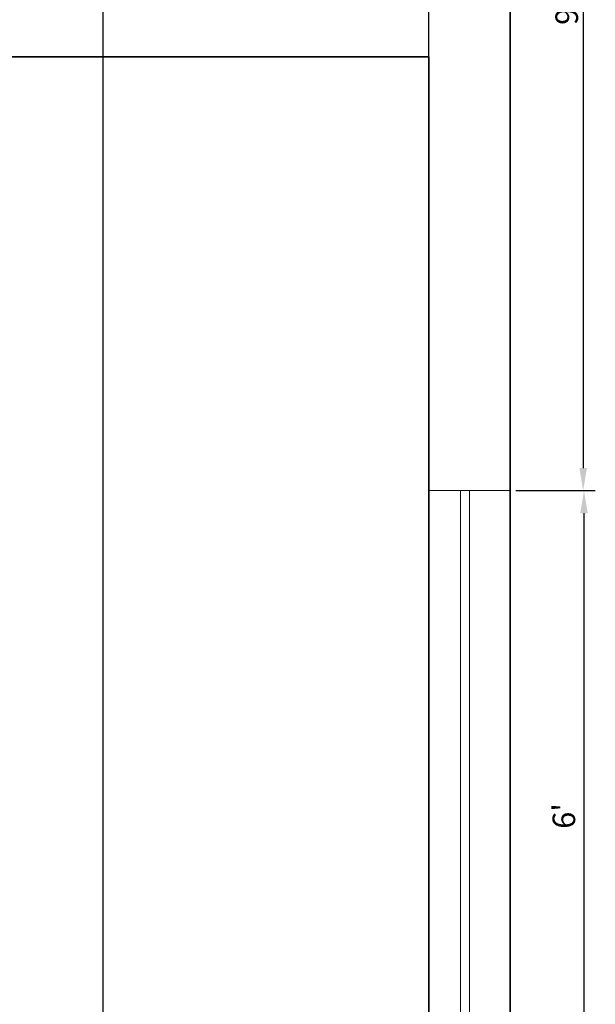
# Model space of a CAD drawing. Units: inches. Extents: x 1624 to 3956, y 1589 to 5028.
# Tile 14 of 16: x 2046 to 2110, y 2317 to 2426. Entities that reach past the tile are written whole.
import ezdxf

# ---------------------------------------------------------------- set-up
doc = ezdxf.new("R2010")
doc.units = ezdxf.units.IN
for name, color, linetype, lineweight in [('A-ANNO-DIMS', 2, 'Continuous', 13), ('A-GLAZ', 4, 'Continuous', 18), ('A-WALL', 7, 'Continuous', 35)]:
    doc.layers.add(name, color=color, linetype=linetype, lineweight=lineweight)
doc.styles.get("Standard").update_dxf_attribs({"font": 'arial.ttf'})
doc.dimstyles.new('Copy of ISO-25', dxfattribs={"dimtxt": 2.5, "dimasz": 2.5, "dimexe": 1.25, "dimexo": 0.625, "dimtad": 1, "dimdec": 1, "dimlunit": 4, "dimtxsty": 'Standard', "dimcen": 2.5, "dimadec": 0, "dimazin": 0, "dimtfac": 1, "dimtdec": 1, "dimtmove": 0, "dimatfit": 3, "dimfxl": 1, "dimarcsym": 0})

# ---------------------------------------------------------------- blocks, each defined once
blk = doc.blocks.new('*D35')
at = {"layer": 'A-ANNO-DIMS', "color": 0, "lineweight": -2, "transparency": 16777216}
for p, q in [((2101.2, 2486.79), (2109.9, 2486.79)), ((2108.65, 2484.29), (2108.65, 2376.79)), ((2101.2, 2374.29), (2109.9, 2374.29))]:
    blk.add_line(p, q, dxfattribs=at)
at = {"layer": 'A-ANNO-DIMS', "color": 0, "transparency": 16777216}
for points in [[(2108.23, 2484.29), (2109.07, 2484.29), (2108.65, 2486.79)], [(2108.23, 2376.79), (2109.07, 2376.79), (2108.65, 2374.29)]]:
    blk.add_solid(points, dxfattribs=at)
at = {"layer": 'Defpoints', "color": 0, "transparency": 16777216}
for p in [(2100.58, 2486.79), (2100.58, 2374.29), (2108.65, 2374.29)]:
    blk.add_point(p, dxfattribs=at)
at = {"layer": 'A-ANNO-DIMS', "color": 0, "transparency": 16777216, "insert": (2105.08, 2430.54), "char_height": 2.5, "attachment_point": 5, "rotation": 90}
blk.add_mtext('9\'-4{\\H1x;\\S1/2;}"', dxfattribs=at)
blk = doc.blocks.new('*D36')
at = {"layer": 'A-ANNO-DIMS', "color": 0, "lineweight": -2, "transparency": 16777216}
for p, q in [((2101.2, 2374.29), (2109.99, 2374.29)), ((2108.74, 2371.79), (2108.74, 2304.79)), ((2101.2, 2302.29), (2109.99, 2302.29))]:
    blk.add_line(p, q, dxfattribs=at)
at = {"layer": 'A-ANNO-DIMS', "color": 0, "transparency": 16777216}
for points in [[(2108.33, 2371.79), (2109.16, 2371.79), (2108.74, 2374.29)], [(2108.33, 2304.79), (2109.16, 2304.79), (2108.74, 2302.29)]]:
    blk.add_solid(points, dxfattribs=at)
at = {"layer": 'Defpoints', "color": 0, "transparency": 16777216}
for p in [(2100.58, 2374.29), (2100.58, 2302.29), (2108.74, 2302.29)]:
    blk.add_point(p, dxfattribs=at)
at = {"layer": 'A-ANNO-DIMS', "color": 0, "transparency": 16777216, "insert": (2106.84, 2338.29), "char_height": 2.5, "attachment_point": 5, "rotation": 90}
blk.add_mtext("6'", dxfattribs=at)
blk = doc.blocks.new('WINDOW-72IN')
for p, q in [((0, 9), (0, 0)), ((72, 0), (72, 9)), ((0, 4.5), (72, 4.5)), ((0, 3.5), (72, 3.5))]:
    blk.add_line(p, q)
blk = doc.blocks.new('*D79')
at = {"layer": 'A-ANNO-DIMS', "color": 0, "lineweight": -2, "transparency": 16777216}
for p, q in [((2090.95, 2422.29), (1628.86, 2422.29)), ((1630.11, 2419.79), (1630.11, 2256.79)), ((2090.95, 2254.29), (1628.86, 2254.29))]:
    blk.add_line(p, q, dxfattribs=at)
at = {"layer": 'A-ANNO-DIMS', "color": 0, "transparency": 16777216}
for points in [[(1629.69, 2419.79), (1630.53, 2419.79), (1630.11, 2422.29)], [(1629.69, 2256.79), (1630.53, 2256.79), (1630.11, 2254.29)]]:
    blk.add_solid(points, dxfattribs=at)
at = {"layer": 'Defpoints', "color": 0, "transparency": 16777216}
for p in [(2091.58, 2422.29), (1630.11, 2254.29), (2091.58, 2254.29)]:
    blk.add_point(p, dxfattribs=at)
at = {"layer": 'A-ANNO-DIMS', "color": 0, "transparency": 16777216, "insert": (1628.21, 2338.29), "char_height": 2.5, "attachment_point": 5, "rotation": 90}
blk.add_mtext('14\'-0"', dxfattribs=at)
blk = doc.blocks.new('*D81')
at = {"layer": 'A-ANNO-DIMS', "color": 0, "lineweight": -2, "transparency": 16777216}
for p, q in [((1951.58, 2254.92), (1951.58, 2612.84)), ((2091.58, 2254.92), (2091.58, 2612.84)), ((1954.08, 2611.59), (2089.08, 2611.59))]:
    blk.add_line(p, q, dxfattribs=at)
at = {"layer": 'A-ANNO-DIMS', "color": 0, "transparency": 16777216}
for points in [[(1954.08, 2612.01), (1954.08, 2611.18), (1951.58, 2611.59)], [(2089.08, 2612.01), (2089.08, 2611.18), (2091.58, 2611.59)]]:
    blk.add_solid(points, dxfattribs=at)
at = {"layer": 'Defpoints', "color": 0, "transparency": 16777216}
for p in [(2091.58, 2611.59), (1951.58, 2254.29), (2091.58, 2254.29)]:
    blk.add_point(p, dxfattribs=at)
at = {"layer": 'A-ANNO-DIMS', "color": 0, "transparency": 16777216, "insert": (2021.58, 2613.5), "char_height": 2.5, "attachment_point": 5}
blk.add_mtext('11\'-8"', dxfattribs=at)
blk = doc.blocks.new('*D90')
at = {"layer": 'A-ANNO-DIMS', "color": 0, "lineweight": -2, "transparency": 16777216}
for p, q in [((2019.58, 1941.92), (2019.58, 2612.84)), ((2055.58, 1941.92), (2055.58, 2612.84)), ((2022.08, 2611.59), (2053.08, 2611.59))]:
    blk.add_line(p, q, dxfattribs=at)
at = {"layer": 'A-ANNO-DIMS', "color": 0, "transparency": 16777216}
for points in [[(2022.08, 2612.01), (2022.08, 2611.18), (2019.58, 2611.59)], [(2053.08, 2612.01), (2053.08, 2611.18), (2055.58, 2611.59)]]:
    blk.add_solid(points, dxfattribs=at)
at = {"layer": 'Defpoints', "color": 0, "transparency": 16777216}
for p in [(2055.58, 2611.59), (2019.58, 1941.29), (2055.58, 1941.29)]:
    blk.add_point(p, dxfattribs=at)
at = {"layer": 'A-ANNO-DIMS', "color": 0, "transparency": 16777216, "insert": (2037.58, 2613.5), "char_height": 2.5, "attachment_point": 5}
blk.add_mtext('3\'-0"', dxfattribs=at)

msp = doc.modelspace()

# ---------------------------------------------------------------- linework, layer by layer
at = {"layer": 'A-GLAZ'}
msp.add_line((2100.58, 2374.29), (2100.58, 2302.29), dxfattribs=at)
at = {"layer": 'A-WALL'}
for p, q in [((2100.58, 2486.79), (2100.58, 2374.29)), ((2091.58, 2422.29), (1951.58, 2422.29)), ((2091.58, 2422.29), (2091.58, 2254.29)), ((2091.58, 2422.29), (2091.58, 2374.29)), ((2100.58, 2374.29), (2100.58, 2254.29))]:
    msp.add_line(p, q, dxfattribs=at)

# ---------------------------------------------------------------- block references
at = {"layer": 'A-GLAZ', "rotation": 270}
msp.add_blockref('WINDOW-72IN', (2091.58, 2374.29), dxfattribs=at)

# ---------------------------------------------------------------- dimensions: what is measured, and where the dimension line sits
at = {"layer": 'A-ANNO-DIMS'}
for base, p1, p2, picture, middle in [((2091.58, 2611.59), (1951.58, 2254.29), (2091.58, 2254.29), '*D81', (2021.58, 2613.5)), ((2055.58, 2611.59), (2019.58, 1941.29), (2055.58, 1941.29), '*D90', (2037.58, 2613.5))]:
    dim = msp.add_linear_dim(base=base, p1=p1, p2=p2, dimstyle='Copy of ISO-25', override={"dimdec": 1, "dimlfac": 1, "dimrnd": 0, "dimzin": 1, "dimdsep": 46, "dimlunit": 4, "dimfrac": 2}, dxfattribs=at)
    dim.commit()
    dim.dimension.update_dxf_attribs({"geometry": picture, "text_midpoint": middle})
for base, p1, p2, override, picture, middle in [((2108.65, 2374.29), (2100.58, 2486.79), (2100.58, 2374.29), {"dimclrd": 0, "dimclre": 0, "dimclrt": 0}, '*D35', (2105.08, 2430.54)), ((1630.11, 2254.29), (2091.58, 2422.29), (2091.58, 2254.29), {"dimdec": 1, "dimlfac": 1, "dimrnd": 0, "dimzin": 1, "dimdsep": 46, "dimlunit": 4, "dimfrac": 2}, '*D79', (1628.21, 2338.29)), ((2108.74, 2302.29), (2100.58, 2374.29), (2100.58, 2302.29), {"dimclrd": 0, "dimclre": 0, "dimclrt": 0}, '*D36', (2106.84, 2338.29))]:
    dim = msp.add_linear_dim(base=base, p1=p1, p2=p2, angle=90, dimstyle='Copy of ISO-25', override=override, dxfattribs=at)
    dim.commit()
    dim.dimension.update_dxf_attribs({"geometry": picture, "text_midpoint": middle})

doc.saveas('drawing.dxf')
